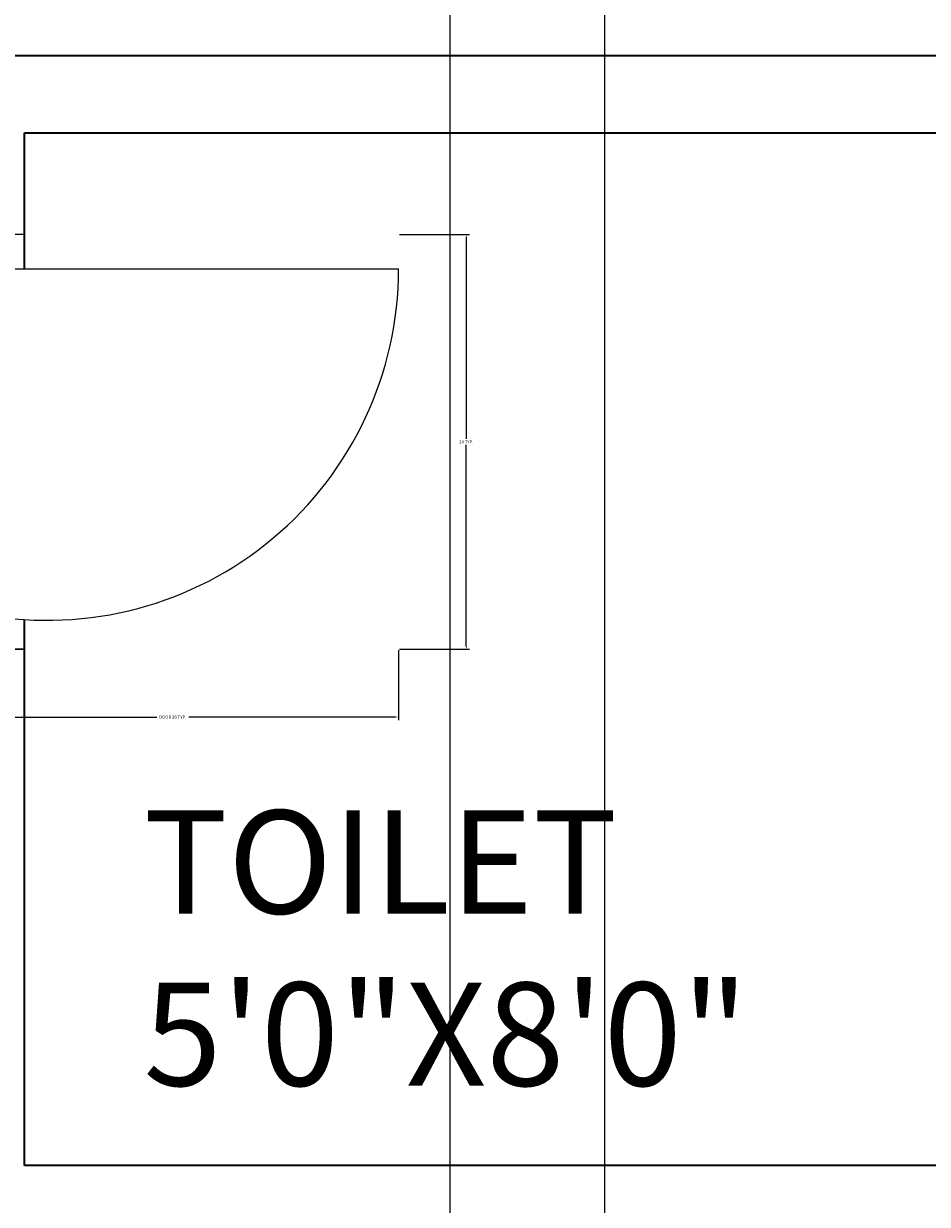
# Model space of a CAD drawing. Units: inches. Extents: x 1088 to 1703, y 668 to 1875.
# Tile 34 of 45: x 1490 to 1542, y 1606 to 1675. Entities that reach past the tile are written whole.
import ezdxf

# ---------------------------------------------------------------- set-up
doc = ezdxf.new("R2010")
doc.units = ezdxf.units.IN
for name, color, linetype, lineweight in [('A-ANNO-DIMS', 2, 'Continuous', 18), ('A-AREA-IDEN', 7, 'Continuous', 18), ('A-DOOR', 4, 'Continuous', 18), ('A-WALL', 7, 'Continuous', 35)]:
    doc.layers.add(name, color=color, linetype=linetype, lineweight=lineweight)
doc.styles.get("Standard").update_dxf_attribs({"font": 'arial.ttf'})
doc.dimstyles.get("Standard").update_dxf_attribs({"dimtxt": 0.18, "dimasz": 0.18, "dimexe": 0.18, "dimexo": 0.0625, "dimgap": 0.09, "dimtad": 0, "dimtih": 1, "dimtoh": 1, "dimdec": 4, "dimzin": 0, "dimdsep": 46, "dimtxsty": 'Standard', "dimcen": 0.09, "dimadec": 0, "dimazin": 0, "dimtfac": 1, "dimtdec": 4, "dimtofl": 0, "dimtmove": 0, "dimatfit": 3, "dimfxl": 1, "dimtolj": 1, "dimtzin": 0, "dimarcsym": 0})

# ---------------------------------------------------------------- blocks, each defined once
blk = doc.blocks.new('DOOR-SWING-24')
for p, q in [((4.5, 24.095), (0, 24.095)), ((0, 24.095), (2.25, 24.095)), ((2.25, 24.095), (2.25, 22.095)), ((2.25, 22.095), (26.25, 22.095)), ((2.25, 0), (2.25, 2)), ((0, 0), (4.5, 0)), ((4.5, 0), (2.25, 0))]:
    blk.add_line(p, q)
blk.add_arc((5.838, 22.095), 20.412, 259.87598, 0)
blk = doc.blocks.new('*D24')
at = {"layer": 'A-ANNO-DIMS', "color": 0, "lineweight": -2, "transparency": 16777216}
for p, q in [((1485.345, 1638.496), (1485.345, 1634.441)), ((1511.595, 1638.496), (1511.595, 1634.441)), ((1485.525, 1634.621), (1497.534, 1634.621)), ((1511.415, 1634.621), (1499.406, 1634.621))]:
    blk.add_line(p, q, dxfattribs=at)
at = {"layer": 'A-ANNO-DIMS', "color": 0, "transparency": 16777216}
for points in [[(1485.525, 1634.651), (1485.525, 1634.591), (1485.345, 1634.621)], [(1511.415, 1634.651), (1511.415, 1634.591), (1511.595, 1634.621)]]:
    blk.add_solid(points, dxfattribs=at)
at = {"layer": 'Defpoints', "color": 0, "transparency": 16777216}
for p in [(1485.345, 1638.558), (1511.595, 1638.558), (1511.595, 1634.621)]:
    blk.add_point(p, dxfattribs=at)
at = {"layer": 'A-ANNO-DIMS', "color": 0, "transparency": 16777216, "insert": (1498.47, 1634.621), "char_height": 0.18, "attachment_point": 5}
blk.add_mtext('\\A1;DOOR 26 TYP.', dxfattribs=at)
blk = doc.blocks.new('*D25')
at = {"layer": 'A-ANNO-DIMS', "color": 0, "lineweight": -2, "transparency": 16777216}
for p, q in [((1511.657, 1662.653), (1515.712, 1662.653)), ((1515.532, 1662.473), (1515.532, 1650.786)), ((1515.532, 1638.738), (1515.532, 1650.425)), ((1511.657, 1638.558), (1515.712, 1638.558))]:
    blk.add_line(p, q, dxfattribs=at)
at = {"layer": 'A-ANNO-DIMS', "color": 0, "transparency": 16777216}
for points in [[(1515.502, 1662.473), (1515.562, 1662.473), (1515.532, 1662.653)], [(1515.502, 1638.738), (1515.562, 1638.738), (1515.532, 1638.558)]]:
    blk.add_solid(points, dxfattribs=at)
at = {"layer": 'Defpoints', "color": 0, "transparency": 16777216}
for p in [(1511.595, 1662.653), (1515.532, 1662.653), (1511.595, 1638.558)]:
    blk.add_point(p, dxfattribs=at)
at = {"layer": 'A-ANNO-DIMS', "color": 0, "transparency": 16777216, "insert": (1515.532, 1650.605), "char_height": 0.18, "attachment_point": 5}
blk.add_mtext('\\A1;24 TYP.', dxfattribs=at)
blk = doc.blocks.new('*D33')
at = {"layer": 'A-ANNO-DIMS', "color": 0, "lineweight": -2, "transparency": 16777216}
for p, q in [((1514.595, 1355.648), (1514.595, 1857.788)), ((1514.775, 1857.608), (1518.946, 1857.608)), ((1523.415, 1857.608), (1519.244, 1857.608)), ((1523.595, 1331.121), (1523.595, 1857.788))]:
    blk.add_line(p, q, dxfattribs=at)
at = {"layer": 'A-ANNO-DIMS', "color": 0, "transparency": 16777216}
for points in [[(1514.775, 1857.638), (1514.775, 1857.578), (1514.595, 1857.608)], [(1523.415, 1857.638), (1523.415, 1857.578), (1523.595, 1857.608)]]:
    blk.add_solid(points, dxfattribs=at)
at = {"layer": 'Defpoints', "color": 0, "transparency": 16777216}
for p in [(1523.595, 1857.608), (1514.595, 1355.585), (1523.595, 1331.058)]:
    blk.add_point(p, dxfattribs=at)
at = {"layer": 'A-ANNO-DIMS', "color": 0, "transparency": 16777216, "insert": (1519.095, 1857.608), "char_height": 0.18, "attachment_point": 5}
blk.add_mtext('\\A1;9', dxfattribs=at)

msp = doc.modelspace()

# ---------------------------------------------------------------- linework, layer by layer
at = {"layer": 'A-WALL'}
for p, q in [((1481.681, 1673.058), (1585.845, 1673.058)), ((1489.845, 1660.653), (1489.845, 1668.558)), ((1489.845, 1668.558), (1585.845, 1668.558)), ((1489.845, 1608.558), (1489.845, 1640.284)), ((1585.845, 1608.558), (1489.845, 1608.558))]:
    msp.add_line(p, q, dxfattribs=at)

# ---------------------------------------------------------------- block references
at = {"layer": 'A-DOOR'}
msp.add_blockref('DOOR-SWING-24', (1485.345, 1638.558), dxfattribs=at)

# ---------------------------------------------------------------- texts
at = {"layer": 'A-AREA-IDEN', "insert": (1496.769, 1629.2), "char_height": 6, "attachment_point": 1}
msp.add_mtext_dynamic_manual_height_columns('TOILET\\P5\'0"X8\'0"', width=133.25429, gutter_width=12.5, heights=[0], dxfattribs=at)

# ---------------------------------------------------------------- dimensions: what is measured, and where the dimension line sits
at = {"layer": 'A-ANNO-DIMS'}
dim = msp.add_linear_dim(base=(1523.595, 1857.608), p1=(1514.595, 1355.585), p2=(1523.595, 1331.058), dimstyle='Standard', override={"dimdec": 0, "dimlfac": 1, "dimrnd": 0, "dimzin": 0, "dimdsep": 46, "dimlunit": 2}, dxfattribs=at)
dim.commit()
dim.dimension.update_dxf_attribs({"geometry": '*D33', "text_midpoint": (1519.095, 1857.608)})
dim = msp.add_linear_dim(base=(1515.532, 1662.653), p1=(1511.595, 1638.558), p2=(1511.595, 1662.653), angle=90, text='<> TYP.', dimstyle='Standard', override={"dimdec": 0, "dimlfac": 1, "dimrnd": 0, "dimzin": 0, "dimdsep": 46, "dimlunit": 2}, dxfattribs=at)
dim.commit()
dim.dimension.update_dxf_attribs({"geometry": '*D25', "text_midpoint": (1515.532, 1650.605)})
dim = msp.add_linear_dim(base=(1511.595, 1634.621), p1=(1485.345, 1638.558), p2=(1511.595, 1638.558), text='DOOR <> TYP.', dimstyle='Standard', override={"dimdec": 0, "dimlfac": 1, "dimrnd": 0, "dimzin": 0, "dimdsep": 46, "dimlunit": 2}, dxfattribs=at)
dim.commit()
dim.dimension.update_dxf_attribs({"geometry": '*D24', "text_midpoint": (1498.47, 1634.621)})

doc.saveas('drawing.dxf')
